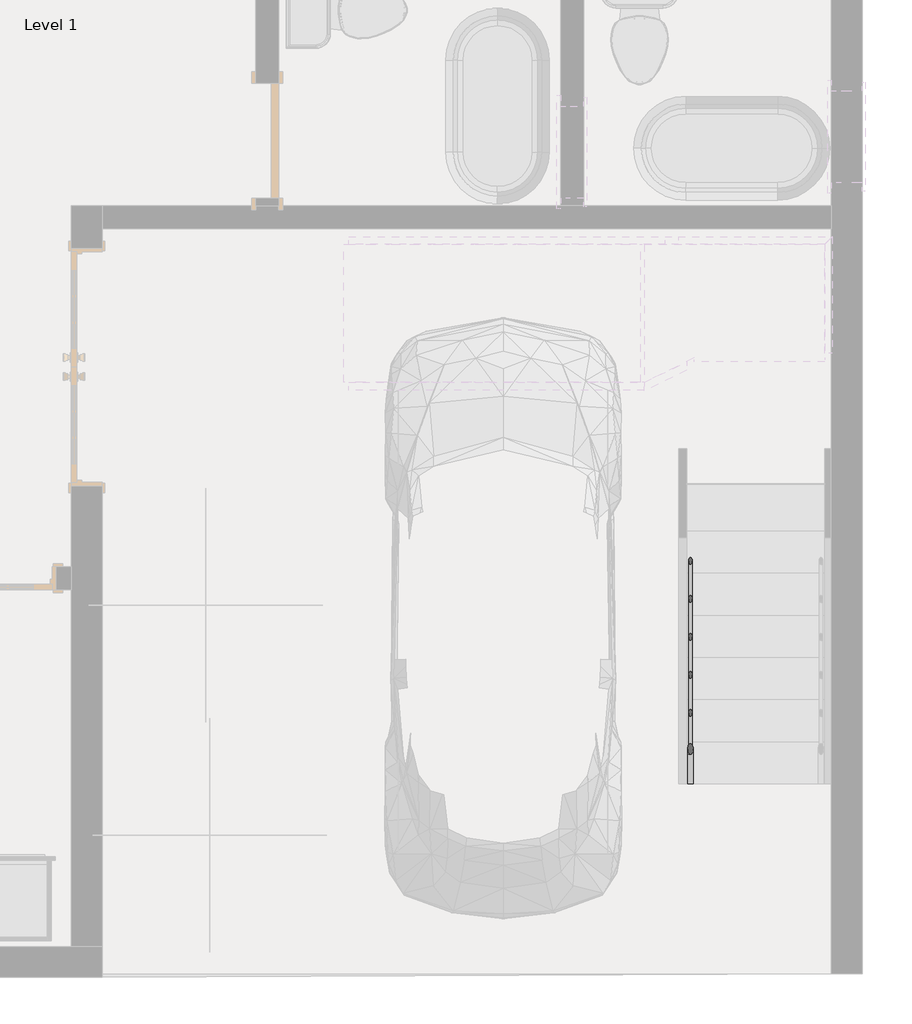
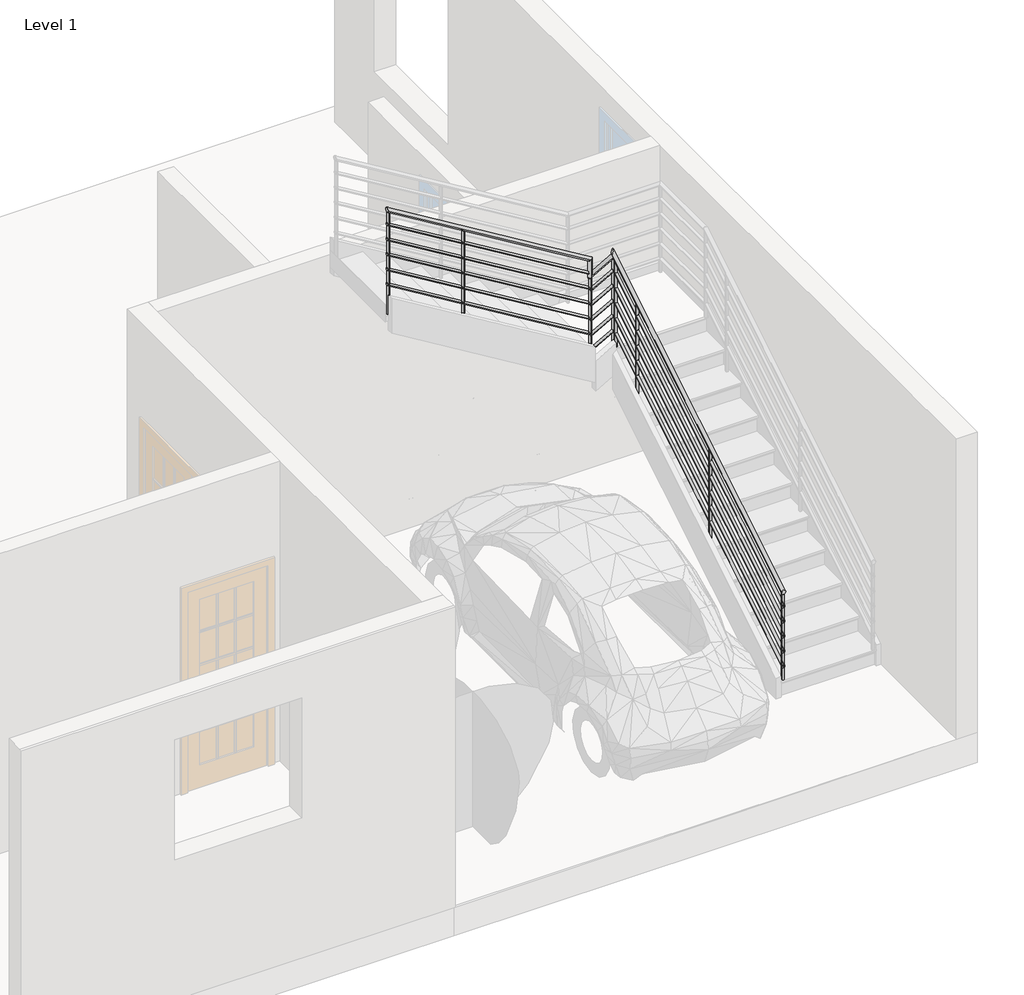
# One storey, part 3 of 5: 1 railing.
"""IFC4 building model written with IfcOpenShell, lengths in millimetres."""

from ifc_helpers import new_model, si_unit, point, frame, frame_2d, origin, place, context, project, spatial, circle_curve, ellipse_curve, trimmed, segment, composite_curve, outline, extrude, element, save
from ifc_brep_helpers import plane_surface, cylinder_surface, advanced_brep

model = new_model("IFC4")

# Units and contexts
model_context = context("Model", 3, world=origin())
ifc_project = project(units=[si_unit("LENGTHUNIT", "METRE", prefix="MILLI")], contexts=[model_context])

# Site, building, storey
site = spatial("IfcSite", under=ifc_project)
building = spatial("IfcBuilding", under=site)
storey = spatial("IfcBuildingStorey", under=building, Name="Level 1", Elevation=0.0)

# Railing
placement = place(None, origin())
element("IfcRailing", 1, ObjectType="Handrail - Pipe", at=placement, inside=storey, context=model_context, shape_type="SolidModel", body=[
    advanced_brep(
    [(-2070.9432736, 3353.09939, 1061.4577857), (-2109.0432736, 3353.09939, 1061.4577857), (-2070.9432736, 6227.2776284, 2803.3839908), (-2109.0432736, 6180.2977008, 2774.9113074)],
    [
        (0, 1, ellipse_curve(frame((-2089.9932736, 3353.09939, 1061.4577857), z_axis=(0.0, -1.0, 0.0), x_axis=(0.0, 0.0, -1.0)), 22.2755476, 19.05)),
        (1, 0, ellipse_curve(frame((-2089.9932736, 3353.09939, 1061.4577857), z_axis=(0.0, -1.0, 0.0), x_axis=(0.0, 0.0, -1.0)), 22.2755476, 19.05)),
        (2, 3, ellipse_curve(frame((-2089.9932736, 6203.7876646, 2789.1476491), z_axis=(-0.8042186020459581, 0.37062014395580417, 0.4646215115741242), x_axis=(-0.5404442051383958, -0.7813013786122838, -0.31223103130674323)), 34.1540054, 19.05)),
        (3, 2, ellipse_curve(frame((-2089.9932736, 6203.7876646, 2789.1476491), z_axis=(-0.8042186020459581, 0.37062014395580417, 0.4646215115741242), x_axis=(-0.5404442051383958, -0.7813013786122838, -0.31223103130674323)), 34.1540054, 19.05)),
        (0, 2),
        (3, 1),
    ],
    [
        plane_surface(frame((-2089.9932736, 3353.09939, 1083.7333333), z_axis=(0.0, -1.0, 0.0), x_axis=(0.0, 0.0, 1.0))),
        plane_surface(frame((-2089.9932736, 6187.918979, 2801.8058115), z_axis=(-0.8042186020459581, 0.37062014395580417, 0.4646215115741242), x_axis=(0.5943336101241835, 0.5015022017683473, 0.6286995319691712))),
        cylinder_surface(frame((-2089.9932736, 3362.9730377, 1067.4418146), z_axis=(0.0, -0.8551978315540538, -0.5183017160932851), x_axis=(-1.0, 0.0, 0.0)), 19.05),
    ],
    [
        (0, [[1, 2]]),
        (1, [[3, 4]]),
        (2, [[-1, 5, -4, 6]]),
        (2, [[-2, -6, -3, -5]]),
    ],
),
    advanced_brep(
    [(-2091.5714529, 6208.3761472, 2758.0166667), (-2116.8877776, 6153.4415743, 2758.0166667), (-2409.12329, 6052.0104202, 2758.0166667), (-2392.2923116, 6017.8296044, 2758.0166667)],
    [
        (0, 1, ellipse_curve(frame((-2104.2296153, 6180.9088608, 2758.0166667), z_axis=(0.8042186020459581, -0.37062014395580417, -0.4646215115741242), x_axis=(0.5404442051383956, 0.7813013786122838, 0.31223103130674307)), 34.1540054, 19.05)),
        (1, 0, ellipse_curve(frame((-2104.2296153, 6180.9088608, 2758.0166667), z_axis=(0.8042186020459581, -0.37062014395580417, -0.4646215115741242), x_axis=(0.5404442051383956, 0.7813013786122838, 0.31223103130674307)), 34.1540054, 19.05)),
        (2, 3, ellipse_curve(frame((-2400.7078008, 6034.9200123, 2758.0166667), z_axis=(-0.6343697273857986, -0.31237005134370305, 0.7071067811865476), x_axis=(0.6343697273857984, 0.312370051343703, 0.7071067811865476)), 26.9407684, 19.05)),
        (3, 2, ellipse_curve(frame((-2400.7078008, 6034.9200123, 2758.0166667), z_axis=(-0.6343697273857986, -0.31237005134370305, 0.7071067811865476), x_axis=(0.6343697273857984, 0.312370051343703, 0.7071067811865476)), 26.9407684, 19.05)),
        (0, 2),
        (3, 1),
    ],
    [
        plane_surface(frame((-2089.9932736, 6187.918979, 2777.0666667), z_axis=(0.8042186020459581, -0.37062014395580417, -0.4646215115741242), x_axis=(0.5943336101241835, 0.5015022017683473, 0.6286995319691712))),
        plane_surface(frame((-2383.6173929, 6043.3355015, 2777.0666667), z_axis=(-0.6343697273857987, -0.3123700513437031, 0.7071067811865477), x_axis=(0.7730297853100279, -0.2563395461339441, 0.5802714779406066))),
        cylinder_surface(frame((-2089.9932736, 6187.918979, 2758.0166667), z_axis=(0.8971342720279193, 0.44175796308944487, 0.0), x_axis=(0.44175796308944487, -0.8971342720279193, 0.0)), 19.05),
    ],
    [
        (0, [[1, 2]]),
        (1, [[3, 4]]),
        (2, [[-1, 5, -4, 6]]),
        (2, [[-2, -6, -3, -5]]),
    ],
),
    advanced_brep(
    [(-2409.12329, 6052.0104202, 2758.0166667), (-2392.2923116, 6017.8296044, 2758.0166667), (-2409.12329, 6052.0104202, 2922.9689103), (-2392.2923116, 6017.8296044, 2932.4491184)],
    [
        (0, 1, ellipse_curve(frame((-2400.7078008, 6034.9200123, 2758.0166667), z_axis=(0.6343697273857986, 0.31237005134370305, -0.7071067811865476), x_axis=(-0.6343697273857987, -0.3123700513437031, -0.7071067811865475)), 26.9407684, 19.05)),
        (1, 0, ellipse_curve(frame((-2400.7078008, 6034.9200123, 2758.0166667), z_axis=(0.6343697273857986, 0.31237005134370305, -0.7071067811865476), x_axis=(-0.6343697273857987, -0.3123700513437031, -0.7071067811865475)), 26.9407684, 19.05)),
        (2, 3, ellipse_curve(frame((-2400.7078008, 6034.9200123, 2927.7090143), z_axis=(-0.4907638352133923, 0.0, 0.8712926362862494), x_axis=(-0.8712926362862494, 0.0, -0.49076383521339195)), 21.8640663, 19.05)),
        (3, 2, ellipse_curve(frame((-2400.7078008, 6034.9200123, 2927.7090143), z_axis=(-0.4907638352133923, 0.0, 0.8712926362862494), x_axis=(-0.8712926362862494, 0.0, -0.49076383521339195)), 21.8640663, 19.05)),
        (0, 2),
        (3, 1),
    ],
    [
        plane_surface(frame((-2400.7078008, 6034.9200123, 2758.0166667), z_axis=(0.6343697273857987, 0.3123700513437031, -0.7071067811865477), x_axis=(0.7730297853100279, -0.2563395461339441, 0.5802714779406066))),
        plane_surface(frame((-2400.7078008, 6034.9200123, 2927.7090143), z_axis=(-0.4907638352133923, 0.0, 0.8712926362862494), x_axis=(0.8712926362862494, 0.0, 0.4907638352133923))),
        cylinder_surface(frame((-2400.7078008, 6034.9200123, 2758.0166667), z_axis=(0.0, 0.0, -1.0), x_axis=(0.44175796308944487, -0.8971342720279193, 0.0)), 19.05),
    ],
    [
        (0, [[1, 2]]),
        (1, [[3, 4]]),
        (2, [[-1, 5, -4, 6]]),
        (2, [[-2, -6, -3, -5]]),
    ],
),
    advanced_brep(
    [(-2400.7078008, 6053.9700123, 2927.7090143), (-2400.7078008, 6015.8700123, 2927.7090143), (-4350.5932736, 6053.9700123, 4109.4577857), (-4350.5932736, 6015.8700123, 4109.4577857)],
    [
        (0, 1, ellipse_curve(frame((-2400.7078008, 6034.9200123, 2927.7090143), z_axis=(0.4907638352133923, 0.0, -0.8712926362862494), x_axis=(0.8712926362862492, 0.0, 0.4907638352133924)), 21.8640663, 19.05)),
        (1, 0, ellipse_curve(frame((-2400.7078008, 6034.9200123, 2927.7090143), z_axis=(0.4907638352133923, 0.0, -0.8712926362862494), x_axis=(0.8712926362862492, 0.0, 0.4907638352133924)), 21.8640663, 19.05)),
        (2, 3, ellipse_curve(frame((-4350.5932736, 6034.9200123, 4109.4577857), z_axis=(-1.0, 0.0, 0.0), x_axis=(0.0, 0.0, -1.0)), 22.2755476, 19.05)),
        (3, 2, ellipse_curve(frame((-4350.5932736, 6034.9200123, 4109.4577857), z_axis=(-1.0, 0.0, 0.0), x_axis=(0.0, 0.0, -1.0)), 22.2755476, 19.05)),
        (0, 2),
        (3, 1),
    ],
    [
        plane_surface(frame((-2381.6578008, 6034.9200123, 2938.4391074), z_axis=(0.4907638352133923, 0.0, -0.8712926362862494), x_axis=(0.8712926362862494, 0.0, 0.4907638352133923))),
        plane_surface(frame((-4350.5932736, 6034.9200123, 4131.7333333), z_axis=(-1.0, 0.0, 0.0), x_axis=(0.0, -1.0, 0.0))),
        cylinder_surface(frame((-2391.5314485, 6034.9200123, 2922.1475887), z_axis=(0.855197831554054, 0.0, -0.5183017160932848), x_axis=(0.0, -1.0, 0.0)), 19.05),
    ],
    [
        (0, [[1, 2]]),
        (1, [[3, 4]]),
        (2, [[-1, 5, -4, 6]]),
        (2, [[-2, -6, -3, -5]]),
    ],
),
    advanced_brep(
    [(-2077.2932736, 3353.09939, 916.4829683), (-2102.6932736, 3353.09939, 916.4829683), (-2077.2932736, 6150.6474924, 2611.9666667), (-2102.6932736, 6150.6474924, 2611.9666667), (-2077.2932736, 6208.3287735, 2611.9666667), (-2102.6932736, 6167.5091845, 2611.9666667), (-2400.7078008, 6049.0761987, 2611.9666667), (-2400.7078008, 6020.7638259, 2611.9666667)],
    [
        (0, 1, ellipse_curve(frame((-2089.9932736, 3353.09939, 916.4829683), z_axis=(0.0, -1.0, 0.0), x_axis=(0.0, 0.0, -1.0)), 14.8503651, 12.7)),
        (1, 0, ellipse_curve(frame((-2089.9932736, 3353.09939, 916.4829683), z_axis=(0.0, -1.0, 0.0), x_axis=(0.0, 0.0, -1.0)), 14.8503651, 12.7)),
        (0, 2),
        (2, 3, ellipse_curve(frame((-2089.9932736, 6150.6474924, 2611.9666667), z_axis=(0.0, -0.9631193673564181, -0.26907449567540415), x_axis=(0.0, 0.26907449567540453, -0.9631193673564179)), 13.1863198, 12.7)),
        (3, 1),
        (3, 2, ellipse_curve(frame((-2089.9932736, 6150.6474924, 2611.9666667), z_axis=(0.0, -0.9631193673564181, -0.26907449567540415), x_axis=(0.0, 0.26907449567540453, -0.9631193673564179)), 13.1863198, 12.7)),
        (2, 4),
        (4, 5, ellipse_curve(frame((-2089.9932736, 6187.918979, 2611.9666667), z_axis=(0.849045924284854, -0.5283190498697528, 0.0), x_axis=(-0.5283190498697528, -0.8490459242848537, 0.0)), 24.0385048, 12.7)),
        (5, 3),
        (5, 4, ellipse_curve(frame((-2089.9932736, 6187.918979, 2611.9666667), z_axis=(0.849045924284854, -0.5283190498697528, 0.0), x_axis=(-0.5283190498697528, -0.8490459242848537, 0.0)), 24.0385048, 12.7)),
        (6, 7, ellipse_curve(frame((-2400.7078008, 6034.9200123, 2611.9666667), z_axis=(-1.0, 0.0, 0.0), x_axis=(0.0, 1.0, 0.0)), 14.1561864, 12.7)),
        (7, 6, ellipse_curve(frame((-2400.7078008, 6034.9200123, 2611.9666667), z_axis=(-1.0, 0.0, 0.0), x_axis=(0.0, 1.0, 0.0)), 14.1561864, 12.7)),
        (4, 6),
        (7, 5),
    ],
    [
        plane_surface(frame((-2089.9932736, 3353.09939, 931.3333333), z_axis=(0.0, -1.0, 0.0), x_axis=(0.0, 0.0, 1.0))),
        cylinder_surface(frame((-2089.9932736, 3359.6818218, 920.4723209), z_axis=(0.0, -0.8551978315540539, -0.518301716093285), x_axis=(-1.0, 0.0, 0.0)), 12.7),
        cylinder_surface(frame((-2089.9932736, 6147.09939, 2611.9666667), z_axis=(0.0, -1.0, 0.0), x_axis=(-1.0, 0.0, 0.0)), 12.7),
        plane_surface(frame((-2400.7078008, 6034.9200123, 2624.6666667), z_axis=(-1.0, 0.0, 0.0), x_axis=(0.0, -1.0, 0.0))),
        cylinder_surface(frame((-2089.9932736, 6187.918979, 2611.9666667), z_axis=(0.8971342720279194, 0.4417579630894449, 0.0), x_axis=(0.4417579630894449, -0.8971342720279194, 0.0)), 12.7),
    ],
    [
        (0, [[1, 2]]),
        (1, [[-1, 3, 4, 5]]),
        (1, [[-2, -5, 6, -3]]),
        (2, [[-4, 7, 8, 9]]),
        (2, [[-6, -9, 10, -7]]),
        (3, [[11, 12]]),
        (4, [[-8, 13, -12, 14]]),
        (4, [[-10, -14, -11, -13]]),
    ],
),
    advanced_brep(
    [(-2400.7078008, 6047.6200123, 2782.7341969), (-2400.7078008, 6022.2200123, 2782.7341969), (-4350.5932736, 6047.6200123, 3964.4829683), (-4350.5932736, 6022.2200123, 3964.4829683)],
    [
        (0, 1, ellipse_curve(frame((-2400.7078008, 6034.9200123, 2782.7341969), z_axis=(1.0, 0.0, 0.0), x_axis=(0.0, 0.0, -1.0)), 14.8503651, 12.7)),
        (1, 0, ellipse_curve(frame((-2400.7078008, 6034.9200123, 2782.7341969), z_axis=(1.0, 0.0, 0.0), x_axis=(0.0, 0.0, -1.0)), 14.8503651, 12.7)),
        (2, 3, ellipse_curve(frame((-4350.5932736, 6034.9200123, 3964.4829683), z_axis=(-1.0, 0.0, 0.0), x_axis=(0.0, 0.0, -1.0)), 14.8503651, 12.7)),
        (3, 2, ellipse_curve(frame((-4350.5932736, 6034.9200123, 3964.4829683), z_axis=(-1.0, 0.0, 0.0), x_axis=(0.0, 0.0, -1.0)), 14.8503651, 12.7)),
        (0, 2),
        (3, 1),
    ],
    [
        plane_surface(frame((-2400.7078008, 6034.9200123, 2797.5845619), z_axis=(1.0, 0.0, 0.0), x_axis=(0.0, -1.0, 0.0))),
        plane_surface(frame((-4350.5932736, 6034.9200123, 3979.3333333), z_axis=(-1.0, 0.0, 0.0), x_axis=(0.0, -1.0, 0.0))),
        cylinder_surface(frame((-2407.2902326, 6034.9200123, 2786.7235495), z_axis=(0.855197831554054, 0.0, -0.5183017160932848), x_axis=(0.0, -1.0, 0.0)), 12.7),
    ],
    [
        (0, [[1, 2]]),
        (1, [[3, 4]]),
        (2, [[-1, 5, -4, 6]]),
        (2, [[-2, -6, -3, -5]]),
    ],
),
    advanced_brep(
    [(-2077.2932736, 3353.09939, 764.0829683), (-2102.6932736, 3353.09939, 764.0829683), (-2077.2932736, 6150.6474924, 2459.5666667), (-2102.6932736, 6150.6474924, 2459.5666667), (-2077.2932736, 6208.3287735, 2459.5666667), (-2102.6932736, 6167.5091845, 2459.5666667), (-2400.7078008, 6049.0761987, 2459.5666667), (-2400.7078008, 6020.7638259, 2459.5666667)],
    [
        (0, 1, ellipse_curve(frame((-2089.9932736, 3353.09939, 764.0829683), z_axis=(0.0, -1.0, 0.0), x_axis=(0.0, 0.0, -1.0)), 14.8503651, 12.7)),
        (1, 0, ellipse_curve(frame((-2089.9932736, 3353.09939, 764.0829683), z_axis=(0.0, -1.0, 0.0), x_axis=(0.0, 0.0, -1.0)), 14.8503651, 12.7)),
        (0, 2),
        (2, 3, ellipse_curve(frame((-2089.9932736, 6150.6474924, 2459.5666667), z_axis=(0.0, -0.9631193673564181, -0.26907449567540415), x_axis=(0.0, 0.26907449567540453, -0.9631193673564179)), 13.1863198, 12.7)),
        (3, 1),
        (3, 2, ellipse_curve(frame((-2089.9932736, 6150.6474924, 2459.5666667), z_axis=(0.0, -0.9631193673564181, -0.26907449567540415), x_axis=(0.0, 0.26907449567540453, -0.9631193673564179)), 13.1863198, 12.7)),
        (2, 4),
        (4, 5, ellipse_curve(frame((-2089.9932736, 6187.918979, 2459.5666667), z_axis=(0.849045924284854, -0.5283190498697528, 0.0), x_axis=(-0.5283190498697528, -0.8490459242848537, 0.0)), 24.0385048, 12.7)),
        (5, 3),
        (5, 4, ellipse_curve(frame((-2089.9932736, 6187.918979, 2459.5666667), z_axis=(0.849045924284854, -0.5283190498697528, 0.0), x_axis=(-0.5283190498697528, -0.8490459242848537, 0.0)), 24.0385048, 12.7)),
        (6, 7, ellipse_curve(frame((-2400.7078008, 6034.9200123, 2459.5666667), z_axis=(-1.0, 0.0, 0.0), x_axis=(0.0, 1.0, 0.0)), 14.1561864, 12.7)),
        (7, 6, ellipse_curve(frame((-2400.7078008, 6034.9200123, 2459.5666667), z_axis=(-1.0, 0.0, 0.0), x_axis=(0.0, 1.0, 0.0)), 14.1561864, 12.7)),
        (4, 6),
        (7, 5),
    ],
    [
        plane_surface(frame((-2089.9932736, 3353.09939, 778.9333333), z_axis=(0.0, -1.0, 0.0), x_axis=(0.0, 0.0, 1.0))),
        cylinder_surface(frame((-2089.9932736, 3359.6818218, 768.0723209), z_axis=(0.0, -0.8551978315540539, -0.518301716093285), x_axis=(-1.0, 0.0, 0.0)), 12.7),
        cylinder_surface(frame((-2089.9932736, 6147.09939, 2459.5666667), z_axis=(0.0, -1.0, 0.0), x_axis=(-1.0, 0.0, 0.0)), 12.7),
        plane_surface(frame((-2400.7078008, 6034.9200123, 2472.2666667), z_axis=(-1.0, 0.0, 0.0), x_axis=(0.0, -1.0, 0.0))),
        cylinder_surface(frame((-2089.9932736, 6187.918979, 2459.5666667), z_axis=(0.8971342720279194, 0.4417579630894449, 0.0), x_axis=(0.4417579630894449, -0.8971342720279194, 0.0)), 12.7),
    ],
    [
        (0, [[1, 2]]),
        (1, [[-1, 3, 4, 5]]),
        (1, [[-2, -5, 6, -3]]),
        (2, [[-4, 7, 8, 9]]),
        (2, [[-6, -9, 10, -7]]),
        (3, [[11, 12]]),
        (4, [[-8, 13, -12, 14]]),
        (4, [[-10, -14, -11, -13]]),
    ],
),
    advanced_brep(
    [(-2400.7078008, 6047.6200123, 2630.3341969), (-2400.7078008, 6022.2200123, 2630.3341969), (-4350.5932736, 6047.6200123, 3812.0829683), (-4350.5932736, 6022.2200123, 3812.0829683)],
    [
        (0, 1, ellipse_curve(frame((-2400.7078008, 6034.9200123, 2630.3341969), z_axis=(1.0, 0.0, 0.0), x_axis=(0.0, 0.0, -1.0)), 14.8503651, 12.7)),
        (1, 0, ellipse_curve(frame((-2400.7078008, 6034.9200123, 2630.3341969), z_axis=(1.0, 0.0, 0.0), x_axis=(0.0, 0.0, -1.0)), 14.8503651, 12.7)),
        (2, 3, ellipse_curve(frame((-4350.5932736, 6034.9200123, 3812.0829683), z_axis=(-1.0, 0.0, 0.0), x_axis=(0.0, 0.0, -1.0)), 14.8503651, 12.7)),
        (3, 2, ellipse_curve(frame((-4350.5932736, 6034.9200123, 3812.0829683), z_axis=(-1.0, 0.0, 0.0), x_axis=(0.0, 0.0, -1.0)), 14.8503651, 12.7)),
        (0, 2),
        (3, 1),
    ],
    [
        plane_surface(frame((-2400.7078008, 6034.9200123, 2645.1845619), z_axis=(1.0, 0.0, 0.0), x_axis=(0.0, -1.0, 0.0))),
        plane_surface(frame((-4350.5932736, 6034.9200123, 3826.9333333), z_axis=(-1.0, 0.0, 0.0), x_axis=(0.0, -1.0, 0.0))),
        cylinder_surface(frame((-2407.2902326, 6034.9200123, 2634.3235495), z_axis=(0.855197831554054, 0.0, -0.5183017160932848), x_axis=(0.0, -1.0, 0.0)), 12.7),
    ],
    [
        (0, [[1, 2]]),
        (1, [[3, 4]]),
        (2, [[-1, 5, -4, 6]]),
        (2, [[-2, -6, -3, -5]]),
    ],
),
    advanced_brep(
    [(-2077.2932736, 3353.09939, 611.6829683), (-2102.6932736, 3353.09939, 611.6829683), (-2077.2932736, 6150.6474924, 2307.1666667), (-2102.6932736, 6150.6474924, 2307.1666667), (-2077.2932736, 6208.3287735, 2307.1666667), (-2102.6932736, 6167.5091845, 2307.1666667), (-2400.7078008, 6049.0761987, 2307.1666667), (-2400.7078008, 6020.7638259, 2307.1666667)],
    [
        (0, 1, ellipse_curve(frame((-2089.9932736, 3353.09939, 611.6829683), z_axis=(0.0, -1.0, 0.0), x_axis=(0.0, 0.0, -1.0)), 14.8503651, 12.7)),
        (1, 0, ellipse_curve(frame((-2089.9932736, 3353.09939, 611.6829683), z_axis=(0.0, -1.0, 0.0), x_axis=(0.0, 0.0, -1.0)), 14.8503651, 12.7)),
        (0, 2),
        (2, 3, ellipse_curve(frame((-2089.9932736, 6150.6474924, 2307.1666667), z_axis=(0.0, -0.9631193673564181, -0.26907449567540415), x_axis=(0.0, 0.26907449567540453, -0.9631193673564179)), 13.1863198, 12.7)),
        (3, 1),
        (3, 2, ellipse_curve(frame((-2089.9932736, 6150.6474924, 2307.1666667), z_axis=(0.0, -0.9631193673564181, -0.26907449567540415), x_axis=(0.0, 0.26907449567540453, -0.9631193673564179)), 13.1863198, 12.7)),
        (2, 4),
        (4, 5, ellipse_curve(frame((-2089.9932736, 6187.918979, 2307.1666667), z_axis=(0.849045924284854, -0.5283190498697528, 0.0), x_axis=(-0.5283190498697528, -0.8490459242848537, 0.0)), 24.0385048, 12.7)),
        (5, 3),
        (5, 4, ellipse_curve(frame((-2089.9932736, 6187.918979, 2307.1666667), z_axis=(0.849045924284854, -0.5283190498697528, 0.0), x_axis=(-0.5283190498697528, -0.8490459242848537, 0.0)), 24.0385048, 12.7)),
        (6, 7, ellipse_curve(frame((-2400.7078008, 6034.9200123, 2307.1666667), z_axis=(-1.0, 0.0, 0.0), x_axis=(0.0, 1.0, 0.0)), 14.1561864, 12.7)),
        (7, 6, ellipse_curve(frame((-2400.7078008, 6034.9200123, 2307.1666667), z_axis=(-1.0, 0.0, 0.0), x_axis=(0.0, 1.0, 0.0)), 14.1561864, 12.7)),
        (4, 6),
        (7, 5),
    ],
    [
        plane_surface(frame((-2089.9932736, 3353.09939, 626.5333333), z_axis=(0.0, -1.0, 0.0), x_axis=(0.0, 0.0, 1.0))),
        cylinder_surface(frame((-2089.9932736, 3359.6818218, 615.6723209), z_axis=(0.0, -0.8551978315540539, -0.518301716093285), x_axis=(-1.0, 0.0, 0.0)), 12.7),
        cylinder_surface(frame((-2089.9932736, 6147.09939, 2307.1666667), z_axis=(0.0, -1.0, 0.0), x_axis=(-1.0, 0.0, 0.0)), 12.7),
        plane_surface(frame((-2400.7078008, 6034.9200123, 2319.8666667), z_axis=(-1.0, 0.0, 0.0), x_axis=(0.0, -1.0, 0.0))),
        cylinder_surface(frame((-2089.9932736, 6187.918979, 2307.1666667), z_axis=(0.8971342720279194, 0.4417579630894449, 0.0), x_axis=(0.4417579630894449, -0.8971342720279194, 0.0)), 12.7),
    ],
    [
        (0, [[1, 2]]),
        (1, [[-1, 3, 4, 5]]),
        (1, [[-2, -5, 6, -3]]),
        (2, [[-4, 7, 8, 9]]),
        (2, [[-6, -9, 10, -7]]),
        (3, [[11, 12]]),
        (4, [[-8, 13, -12, 14]]),
        (4, [[-10, -14, -11, -13]]),
    ],
),
    advanced_brep(
    [(-2400.7078008, 6047.6200123, 2477.9341969), (-2400.7078008, 6022.2200123, 2477.9341969), (-4350.5932736, 6047.6200123, 3659.6829683), (-4350.5932736, 6022.2200123, 3659.6829683)],
    [
        (0, 1, ellipse_curve(frame((-2400.7078008, 6034.9200123, 2477.9341969), z_axis=(1.0, 0.0, 0.0), x_axis=(0.0, 0.0, -1.0)), 14.8503651, 12.7)),
        (1, 0, ellipse_curve(frame((-2400.7078008, 6034.9200123, 2477.9341969), z_axis=(1.0, 0.0, 0.0), x_axis=(0.0, 0.0, -1.0)), 14.8503651, 12.7)),
        (2, 3, ellipse_curve(frame((-4350.5932736, 6034.9200123, 3659.6829683), z_axis=(-1.0, 0.0, 0.0), x_axis=(0.0, 0.0, -1.0)), 14.8503651, 12.7)),
        (3, 2, ellipse_curve(frame((-4350.5932736, 6034.9200123, 3659.6829683), z_axis=(-1.0, 0.0, 0.0), x_axis=(0.0, 0.0, -1.0)), 14.8503651, 12.7)),
        (0, 2),
        (3, 1),
    ],
    [
        plane_surface(frame((-2400.7078008, 6034.9200123, 2492.7845619), z_axis=(1.0, 0.0, 0.0), x_axis=(0.0, -1.0, 0.0))),
        plane_surface(frame((-4350.5932736, 6034.9200123, 3674.5333333), z_axis=(-1.0, 0.0, 0.0), x_axis=(0.0, -1.0, 0.0))),
        cylinder_surface(frame((-2407.2902326, 6034.9200123, 2481.9235495), z_axis=(0.855197831554054, 0.0, -0.5183017160932848), x_axis=(0.0, -1.0, 0.0)), 12.7),
    ],
    [
        (0, [[1, 2]]),
        (1, [[3, 4]]),
        (2, [[-1, 5, -4, 6]]),
        (2, [[-2, -6, -3, -5]]),
    ],
),
    advanced_brep(
    [(-2077.2932736, 3353.09939, 459.2829683), (-2102.6932736, 3353.09939, 459.2829683), (-2077.2932736, 6150.6474924, 2154.7666667), (-2102.6932736, 6150.6474924, 2154.7666667), (-2077.2932736, 6208.3287735, 2154.7666667), (-2102.6932736, 6167.5091845, 2154.7666667), (-2400.7078008, 6049.0761987, 2154.7666667), (-2400.7078008, 6020.7638259, 2154.7666667)],
    [
        (0, 1, ellipse_curve(frame((-2089.9932736, 3353.09939, 459.2829683), z_axis=(0.0, -1.0, 0.0), x_axis=(0.0, 0.0, -1.0)), 14.8503651, 12.7)),
        (1, 0, ellipse_curve(frame((-2089.9932736, 3353.09939, 459.2829683), z_axis=(0.0, -1.0, 0.0), x_axis=(0.0, 0.0, -1.0)), 14.8503651, 12.7)),
        (0, 2),
        (2, 3, ellipse_curve(frame((-2089.9932736, 6150.6474924, 2154.7666667), z_axis=(0.0, -0.9631193673564181, -0.26907449567540415), x_axis=(0.0, 0.26907449567540453, -0.9631193673564179)), 13.1863198, 12.7)),
        (3, 1),
        (3, 2, ellipse_curve(frame((-2089.9932736, 6150.6474924, 2154.7666667), z_axis=(0.0, -0.9631193673564181, -0.26907449567540415), x_axis=(0.0, 0.26907449567540453, -0.9631193673564179)), 13.1863198, 12.7)),
        (2, 4),
        (4, 5, ellipse_curve(frame((-2089.9932736, 6187.918979, 2154.7666667), z_axis=(0.849045924284854, -0.5283190498697528, 0.0), x_axis=(-0.5283190498697528, -0.8490459242848537, 0.0)), 24.0385048, 12.7)),
        (5, 3),
        (5, 4, ellipse_curve(frame((-2089.9932736, 6187.918979, 2154.7666667), z_axis=(0.849045924284854, -0.5283190498697528, 0.0), x_axis=(-0.5283190498697528, -0.8490459242848537, 0.0)), 24.0385048, 12.7)),
        (6, 7, ellipse_curve(frame((-2400.7078008, 6034.9200123, 2154.7666667), z_axis=(-1.0, 0.0, 0.0), x_axis=(0.0, 1.0, 0.0)), 14.1561864, 12.7)),
        (7, 6, ellipse_curve(frame((-2400.7078008, 6034.9200123, 2154.7666667), z_axis=(-1.0, 0.0, 0.0), x_axis=(0.0, 1.0, 0.0)), 14.1561864, 12.7)),
        (4, 6),
        (7, 5),
    ],
    [
        plane_surface(frame((-2089.9932736, 3353.09939, 474.1333333), z_axis=(0.0, -1.0, 0.0), x_axis=(0.0, 0.0, 1.0))),
        cylinder_surface(frame((-2089.9932736, 3359.6818218, 463.2723209), z_axis=(0.0, -0.8551978315540539, -0.518301716093285), x_axis=(-1.0, 0.0, 0.0)), 12.7),
        cylinder_surface(frame((-2089.9932736, 6147.09939, 2154.7666667), z_axis=(0.0, -1.0, 0.0), x_axis=(-1.0, 0.0, 0.0)), 12.7),
        plane_surface(frame((-2400.7078008, 6034.9200123, 2167.4666667), z_axis=(-1.0, 0.0, 0.0), x_axis=(0.0, -1.0, 0.0))),
        cylinder_surface(frame((-2089.9932736, 6187.918979, 2154.7666667), z_axis=(0.8971342720279194, 0.4417579630894449, 0.0), x_axis=(0.4417579630894449, -0.8971342720279194, 0.0)), 12.7),
    ],
    [
        (0, [[1, 2]]),
        (1, [[-1, 3, 4, 5]]),
        (1, [[-2, -5, 6, -3]]),
        (2, [[-4, 7, 8, 9]]),
        (2, [[-6, -9, 10, -7]]),
        (3, [[11, 12]]),
        (4, [[-8, 13, -12, 14]]),
        (4, [[-10, -14, -11, -13]]),
    ],
),
    advanced_brep(
    [(-2400.7078008, 6047.6200123, 2325.5341969), (-2400.7078008, 6022.2200123, 2325.5341969), (-4350.5932736, 6047.6200123, 3507.2829683), (-4350.5932736, 6022.2200123, 3507.2829683)],
    [
        (0, 1, ellipse_curve(frame((-2400.7078008, 6034.9200123, 2325.5341969), z_axis=(1.0, 0.0, 0.0), x_axis=(0.0, 0.0, -1.0)), 14.8503651, 12.7)),
        (1, 0, ellipse_curve(frame((-2400.7078008, 6034.9200123, 2325.5341969), z_axis=(1.0, 0.0, 0.0), x_axis=(0.0, 0.0, -1.0)), 14.8503651, 12.7)),
        (2, 3, ellipse_curve(frame((-4350.5932736, 6034.9200123, 3507.2829683), z_axis=(-1.0, 0.0, 0.0), x_axis=(0.0, 0.0, -1.0)), 14.8503651, 12.7)),
        (3, 2, ellipse_curve(frame((-4350.5932736, 6034.9200123, 3507.2829683), z_axis=(-1.0, 0.0, 0.0), x_axis=(0.0, 0.0, -1.0)), 14.8503651, 12.7)),
        (0, 2),
        (3, 1),
    ],
    [
        plane_surface(frame((-2400.7078008, 6034.9200123, 2340.3845619), z_axis=(1.0, 0.0, 0.0), x_axis=(0.0, -1.0, 0.0))),
        plane_surface(frame((-4350.5932736, 6034.9200123, 3522.1333333), z_axis=(-1.0, 0.0, 0.0), x_axis=(0.0, -1.0, 0.0))),
        cylinder_surface(frame((-2407.2902326, 6034.9200123, 2329.5235495), z_axis=(0.855197831554054, 0.0, -0.5183017160932847), x_axis=(0.0, -1.0, 0.0)), 12.7),
    ],
    [
        (0, [[1, 2]]),
        (1, [[3, 4]]),
        (2, [[-1, 5, -4, 6]]),
        (2, [[-2, -6, -3, -5]]),
    ],
),
    advanced_brep(
    [(-2077.2932736, 3353.09939, 306.8829683), (-2102.6932736, 3353.09939, 306.8829683), (-2077.2932736, 6150.6474924, 2002.3666667), (-2102.6932736, 6150.6474924, 2002.3666667), (-2077.2932736, 6208.3287735, 2002.3666667), (-2102.6932736, 6167.5091845, 2002.3666667), (-2400.7078008, 6049.0761987, 2002.3666667), (-2400.7078008, 6020.7638259, 2002.3666667)],
    [
        (0, 1, ellipse_curve(frame((-2089.9932736, 3353.09939, 306.8829683), z_axis=(0.0, -1.0, 0.0), x_axis=(0.0, 0.0, -1.0)), 14.8503651, 12.7)),
        (1, 0, ellipse_curve(frame((-2089.9932736, 3353.09939, 306.8829683), z_axis=(0.0, -1.0, 0.0), x_axis=(0.0, 0.0, -1.0)), 14.8503651, 12.7)),
        (0, 2),
        (2, 3, ellipse_curve(frame((-2089.9932736, 6150.6474924, 2002.3666667), z_axis=(0.0, -0.9631193673564181, -0.26907449567540415), x_axis=(0.0, 0.26907449567540453, -0.9631193673564179)), 13.1863198, 12.7)),
        (3, 1),
        (3, 2, ellipse_curve(frame((-2089.9932736, 6150.6474924, 2002.3666667), z_axis=(0.0, -0.9631193673564181, -0.26907449567540415), x_axis=(0.0, 0.26907449567540453, -0.9631193673564179)), 13.1863198, 12.7)),
        (2, 4),
        (4, 5, ellipse_curve(frame((-2089.9932736, 6187.918979, 2002.3666667), z_axis=(0.849045924284854, -0.5283190498697528, 0.0), x_axis=(-0.5283190498697528, -0.8490459242848537, 0.0)), 24.0385048, 12.7)),
        (5, 3),
        (5, 4, ellipse_curve(frame((-2089.9932736, 6187.918979, 2002.3666667), z_axis=(0.849045924284854, -0.5283190498697528, 0.0), x_axis=(-0.5283190498697528, -0.8490459242848537, 0.0)), 24.0385048, 12.7)),
        (6, 7, ellipse_curve(frame((-2400.7078008, 6034.9200123, 2002.3666667), z_axis=(-1.0, 0.0, 0.0), x_axis=(0.0, 1.0, 0.0)), 14.1561864, 12.7)),
        (7, 6, ellipse_curve(frame((-2400.7078008, 6034.9200123, 2002.3666667), z_axis=(-1.0, 0.0, 0.0), x_axis=(0.0, 1.0, 0.0)), 14.1561864, 12.7)),
        (4, 6),
        (7, 5),
    ],
    [
        plane_surface(frame((-2089.9932736, 3353.09939, 321.7333333), z_axis=(0.0, -1.0, 0.0), x_axis=(0.0, 0.0, 1.0))),
        cylinder_surface(frame((-2089.9932736, 3359.6818218, 310.8723209), z_axis=(0.0, -0.8551978315540539, -0.518301716093285), x_axis=(-1.0, 0.0, 0.0)), 12.7),
        cylinder_surface(frame((-2089.9932736, 6147.09939, 2002.3666667), z_axis=(0.0, -1.0, 0.0), x_axis=(-1.0, 0.0, 0.0)), 12.7),
        plane_surface(frame((-2400.7078008, 6034.9200123, 2015.0666667), z_axis=(-1.0, 0.0, 0.0), x_axis=(0.0, -1.0, 0.0))),
        cylinder_surface(frame((-2089.9932736, 6187.918979, 2002.3666667), z_axis=(0.8971342720279194, 0.4417579630894449, 0.0), x_axis=(0.4417579630894449, -0.8971342720279194, 0.0)), 12.7),
    ],
    [
        (0, [[1, 2]]),
        (1, [[-1, 3, 4, 5]]),
        (1, [[-2, -5, 6, -3]]),
        (2, [[-4, 7, 8, 9]]),
        (2, [[-6, -9, 10, -7]]),
        (3, [[11, 12]]),
        (4, [[-8, 13, -12, 14]]),
        (4, [[-10, -14, -11, -13]]),
    ],
),
    advanced_brep(
    [(-2400.7078008, 6047.6200123, 2173.1341969), (-2400.7078008, 6022.2200123, 2173.1341969), (-4350.5932736, 6047.6200123, 3354.8829683), (-4350.5932736, 6022.2200123, 3354.8829683)],
    [
        (0, 1, ellipse_curve(frame((-2400.7078008, 6034.9200123, 2173.1341969), z_axis=(1.0, 0.0, 0.0), x_axis=(0.0, 0.0, -1.0)), 14.8503651, 12.7)),
        (1, 0, ellipse_curve(frame((-2400.7078008, 6034.9200123, 2173.1341969), z_axis=(1.0, 0.0, 0.0), x_axis=(0.0, 0.0, -1.0)), 14.8503651, 12.7)),
        (2, 3, ellipse_curve(frame((-4350.5932736, 6034.9200123, 3354.8829683), z_axis=(-1.0, 0.0, 0.0), x_axis=(0.0, 0.0, -1.0)), 14.8503651, 12.7)),
        (3, 2, ellipse_curve(frame((-4350.5932736, 6034.9200123, 3354.8829683), z_axis=(-1.0, 0.0, 0.0), x_axis=(0.0, 0.0, -1.0)), 14.8503651, 12.7)),
        (0, 2),
        (3, 1),
    ],
    [
        plane_surface(frame((-2400.7078008, 6034.9200123, 2187.9845619), z_axis=(1.0, 0.0, 0.0), x_axis=(0.0, -1.0, 0.0))),
        plane_surface(frame((-4350.5932736, 6034.9200123, 3369.7333333), z_axis=(-1.0, 0.0, 0.0), x_axis=(0.0, -1.0, 0.0))),
        cylinder_surface(frame((-2407.2902326, 6034.9200123, 2177.1235495), z_axis=(0.855197831554054, 0.0, -0.5183017160932847), x_axis=(0.0, -1.0, 0.0)), 12.7),
    ],
    [
        (0, [[1, 2]]),
        (1, [[3, 4]]),
        (2, [[-1, 5, -4, 6]]),
        (2, [[-2, -6, -3, -5]]),
    ],
),
    advanced_brep(
    [(-3619.9078008, 6022.2200123, 3644.3425577), (-3619.9078008, 6047.6200123, 3644.3425577), (-3619.9078008, 6047.6200123, 2709.3333333), (-3619.9078008, 6022.2200123, 2709.3333333)],
    [
        (0, 1, ellipse_curve(frame((-3619.9078008, 6034.9200123, 3644.3425577), z_axis=(-0.5183017160932833, 0.0, -0.8551978315540549), x_axis=(-0.855197831554055, 0.0, 0.518301716093283)), 14.8503651, 12.7)),
        (1, 2),
        (2, 3, circle_curve(frame((-3619.9078008, 6034.9200123, 2709.3333333), z_axis=(0.0, 0.0, 1.0), x_axis=(0.0, 1.0, 0.0)), 12.7)),
        (3, 0),
        (3, 2, circle_curve(frame((-3619.9078008, 6034.9200123, 2709.3333333), z_axis=(0.0, 0.0, 1.0), x_axis=(0.0, 1.0, 0.0)), 12.7)),
        (1, 0, ellipse_curve(frame((-3619.9078008, 6034.9200123, 3644.3425577), z_axis=(-0.5183017160932833, 0.0, -0.8551978315540549), x_axis=(-0.855197831554055, 0.0, 0.518301716093283)), 14.8503651, 12.7)),
    ],
    [
        cylinder_surface(frame((-3619.9078008, 6034.9200123, 2480.7333333), z_axis=(0.0, 0.0, 1.0), x_axis=(0.0, 1.0, 0.0)), 12.7),
        plane_surface(frame((-3645.3078008, 6060.3200123, 3659.7364971), z_axis=(0.5183017160932833, 0.0, 0.8551978315540549), x_axis=(0.0, -1.0, 0.0))),
        plane_surface(frame((-3594.5078008, 6060.3200123, 2709.3333333), z_axis=(0.0, 0.0, -1.0), x_axis=(0.0, -1.0, 0.0))),
    ],
    [
        (0, [[1, 2, 3, 4]]),
        (0, [[5, -2, 6, -4]]),
        (1, [[-6, -1]]),
        (2, [[-5, -3]]),
    ],
),
    advanced_brep(
    [(-2102.6932736, 5791.49939, 2517.00042), (-2077.2932736, 5791.49939, 2517.00042), (-2077.2932736, 5791.49939, 1524.0), (-2102.6932736, 5791.49939, 1524.0)],
    [
        (0, 1, ellipse_curve(frame((-2089.9932736, 5791.49939, 2517.00042), z_axis=(0.0, 0.5183017160932833, -0.8551978315540549), x_axis=(0.0, 0.855197831554055, 0.518301716093283)), 14.8503651, 12.7)),
        (1, 2),
        (2, 3, circle_curve(frame((-2089.9932736, 5791.49939, 1524.0), z_axis=(0.0, 0.0, 1.0), x_axis=(1.0, 0.0, 0.0)), 12.7)),
        (3, 0),
        (3, 2, circle_curve(frame((-2089.9932736, 5791.49939, 1524.0), z_axis=(0.0, 0.0, 1.0), x_axis=(1.0, 0.0, 0.0)), 12.7)),
        (1, 0, ellipse_curve(frame((-2089.9932736, 5791.49939, 2517.00042), z_axis=(0.0, 0.5183017160932833, -0.8551978315540549), x_axis=(0.0, 0.855197831554055, 0.518301716093283)), 14.8503651, 12.7)),
    ],
    [
        cylinder_surface(frame((-2089.9932736, 5791.49939, 1295.4), z_axis=(0.0, 0.0, 1.0), x_axis=(1.0, 0.0, 0.0)), 12.7),
        plane_surface(frame((-2064.5932736, 5816.89939, 2532.3943594), z_axis=(0.0, -0.5183017160932833, 0.8551978315540549), x_axis=(-1.0, 0.0, 0.0))),
        plane_surface(frame((-2064.5932736, 5766.09939, 1524.0), z_axis=(0.0, 0.0, -1.0), x_axis=(-1.0, 0.0, 0.0))),
    ],
    [
        (0, [[1, 2, 3, 4]]),
        (0, [[5, -2, 6, -4]]),
        (1, [[-6, -1]]),
        (2, [[-5, -3]]),
    ],
),
    advanced_brep(
    [(-2102.6932736, 4572.29939, 1778.0913291), (-2077.2932736, 4572.29939, 1778.0913291), (-2077.2932736, 4572.29939, 846.6666667), (-2102.6932736, 4572.29939, 846.6666667)],
    [
        (0, 1, ellipse_curve(frame((-2089.9932736, 4572.29939, 1778.0913291), z_axis=(0.0, 0.5183017160932849, -0.8551978315540538), x_axis=(0.0, 0.8551978315540538, 0.518301716093285)), 14.8503651, 12.7)),
        (1, 2),
        (2, 3, circle_curve(frame((-2089.9932736, 4572.29939, 846.6666667), z_axis=(0.0, 0.0, 1.0), x_axis=(1.0, 0.0, 0.0)), 12.7)),
        (3, 0),
        (3, 2, circle_curve(frame((-2089.9932736, 4572.29939, 846.6666667), z_axis=(0.0, 0.0, 1.0), x_axis=(1.0, 0.0, 0.0)), 12.7)),
        (1, 0, ellipse_curve(frame((-2089.9932736, 4572.29939, 1778.0913291), z_axis=(0.0, 0.5183017160932849, -0.8551978315540538), x_axis=(0.0, 0.8551978315540538, 0.518301716093285)), 14.8503651, 12.7)),
    ],
    [
        cylinder_surface(frame((-2089.9932736, 4572.29939, 618.0666667), z_axis=(0.0, 0.0, 1.0), x_axis=(1.0, 0.0, 0.0)), 12.7),
        plane_surface(frame((-2064.5932736, 4597.69939, 1793.4852684), z_axis=(0.0, -0.5183017160932849, 0.8551978315540538), x_axis=(-1.0, 0.0, 0.0))),
        plane_surface(frame((-2064.5932736, 4546.89939, 846.6666667), z_axis=(0.0, 0.0, -1.0), x_axis=(-1.0, 0.0, 0.0))),
    ],
    [
        (0, [[1, 2, 3, 4]]),
        (0, [[5, -2, 6, -4]]),
        (1, [[-6, -1]]),
        (2, [[-5, -3]]),
    ],
),
    extrude(outline(composite_curve([segment(trimmed(circle_curve(frame_2d((-2400.7078008, 6034.9200123)), 12.7), [point((-2400.7078008, 6047.6200123))], [point((-2400.7078008, 6022.2200123))], False, "CARTESIAN"), True, "CONTINUOUS"), segment(trimmed(circle_curve(frame_2d((-2400.7078008, 6034.9200123)), 12.7), [point((-2400.7078008, 6022.2200123))], [point((-2400.7078008, 6047.6200123))], False, "CARTESIAN"), True, "CONTINUOUS")], self_intersect=False)), frame((0.0, 0.0, 2032.0), z_axis=(0.0, 0.0, 1.0), x_axis=(1.0, 0.0, 0.0)), (0.0, 0.0, 1.0), 706.9666667),
    advanced_brep(
    [(-2102.6932736, 6187.918979, 2757.2547163), (-2077.2932736, 6187.918979, 2757.2547163), (-2077.2932736, 6187.918979, 1862.6666667), (-2102.6932736, 6187.918979, 1862.6666667)],
    [
        (0, 1, ellipse_curve(frame((-2089.9932736, 6187.918979, 2757.2547163), z_axis=(0.0, 0.5183017160932833, -0.8551978315540549), x_axis=(0.0, 0.855197831554055, 0.518301716093283)), 14.8503651, 12.7)),
        (1, 2),
        (2, 3, circle_curve(frame((-2089.9932736, 6187.918979, 1862.6666667), z_axis=(0.0, 0.0, 1.0), x_axis=(1.0, 0.0, 0.0)), 12.7)),
        (3, 0),
        (3, 2, circle_curve(frame((-2089.9932736, 6187.918979, 1862.6666667), z_axis=(0.0, 0.0, 1.0), x_axis=(1.0, 0.0, 0.0)), 12.7)),
        (1, 0, ellipse_curve(frame((-2089.9932736, 6187.918979, 2757.2547163), z_axis=(0.0, 0.5183017160932833, -0.8551978315540549), x_axis=(0.0, 0.855197831554055, 0.518301716093283)), 14.8503651, 12.7)),
    ],
    [
        cylinder_surface(frame((-2089.9932736, 6187.918979, 1634.0666667), z_axis=(0.0, 0.0, 1.0), x_axis=(1.0, 0.0, 0.0)), 12.7),
        plane_surface(frame((-2064.5932736, 6213.318979, 2772.6486557), z_axis=(0.0, -0.5183017160932833, 0.8551978315540549), x_axis=(-1.0, 0.0, 0.0))),
        plane_surface(frame((-2064.5932736, 6162.518979, 1862.6666667), z_axis=(0.0, 0.0, -1.0), x_axis=(-1.0, 0.0, 0.0))),
    ],
    [
        (0, [[1, 2, 3, 4]]),
        (0, [[5, -2, 6, -4]]),
        (1, [[-6, -1]]),
        (2, [[-5, -3]]),
    ],
),
    advanced_brep(
    [(-2102.6932736, 6147.09939, 2732.5155715), (-2077.2932736, 6147.09939, 2732.5155715), (-2077.2932736, 6147.09939, 1862.6666667), (-2102.6932736, 6147.09939, 1862.6666667)],
    [
        (0, 1, ellipse_curve(frame((-2089.9932736, 6147.09939, 2732.5155715), z_axis=(0.0, 0.5183017160932817, -0.8551978315540559), x_axis=(0.0, 0.8551978315540559, 0.5183017160932814)), 14.8503651, 12.7)),
        (1, 2),
        (2, 3, circle_curve(frame((-2089.9932736, 6147.09939, 1862.6666667), z_axis=(0.0, 0.0, 1.0), x_axis=(1.0, 0.0, 0.0)), 12.7)),
        (3, 0),
        (3, 2, circle_curve(frame((-2089.9932736, 6147.09939, 1862.6666667), z_axis=(0.0, 0.0, 1.0), x_axis=(1.0, 0.0, 0.0)), 12.7)),
        (1, 0, ellipse_curve(frame((-2089.9932736, 6147.09939, 2732.5155715), z_axis=(0.0, 0.5183017160932817, -0.8551978315540559), x_axis=(0.0, 0.8551978315540559, 0.5183017160932814)), 14.8503651, 12.7)),
    ],
    [
        cylinder_surface(frame((-2089.9932736, 6147.09939, 1634.0666667), z_axis=(0.0, 0.0, 1.0), x_axis=(1.0, 0.0, 0.0)), 12.7),
        plane_surface(frame((-2064.5932736, 6172.49939, 2747.9095109), z_axis=(0.0, -0.5183017160932817, 0.8551978315540559), x_axis=(-1.0, 0.0, 0.0))),
        plane_surface(frame((-2064.5932736, 6121.69939, 1862.6666667), z_axis=(0.0, 0.0, -1.0), x_axis=(-1.0, 0.0, 0.0))),
    ],
    [
        (0, [[1, 2, 3, 4]]),
        (0, [[5, -2, 6, -4]]),
        (1, [[-6, -1]]),
        (2, [[-5, -3]]),
    ],
),
    advanced_brep(
    [(-4337.8932736, 6022.2200123, 4079.4852684), (-4337.8932736, 6047.6200123, 4079.4852684), (-4337.8932736, 6047.6200123, 3048.0), (-4337.8932736, 6022.2200123, 3048.0)],
    [
        (0, 1, ellipse_curve(frame((-4337.8932736, 6034.9200123, 4079.4852684), z_axis=(-0.5183017160932833, 0.0, -0.8551978315540549), x_axis=(-0.855197831554055, 0.0, 0.518301716093283)), 14.8503651, 12.7)),
        (1, 2),
        (2, 3, circle_curve(frame((-4337.8932736, 6034.9200123, 3048.0), z_axis=(0.0, 0.0, 1.0), x_axis=(0.0, 1.0, 0.0)), 12.7)),
        (3, 0),
        (3, 2, circle_curve(frame((-4337.8932736, 6034.9200123, 3048.0), z_axis=(0.0, 0.0, 1.0), x_axis=(0.0, 1.0, 0.0)), 12.7)),
        (1, 0, ellipse_curve(frame((-4337.8932736, 6034.9200123, 4079.4852684), z_axis=(-0.5183017160932833, 0.0, -0.8551978315540549), x_axis=(-0.855197831554055, 0.0, 0.518301716093283)), 14.8503651, 12.7)),
    ],
    [
        cylinder_surface(frame((-4337.8932736, 6034.9200123, 2819.4), z_axis=(0.0, 0.0, 1.0), x_axis=(0.0, 1.0, 0.0)), 12.7),
        plane_surface(frame((-4363.2932736, 6060.3200123, 4094.8792078), z_axis=(0.5183017160932833, 0.0, 0.8551978315540549), x_axis=(0.0, -1.0, 0.0))),
        plane_surface(frame((-4312.4932736, 6060.3200123, 3048.0), z_axis=(0.0, 0.0, -1.0), x_axis=(0.0, -1.0, 0.0))),
    ],
    [
        (0, [[1, 2, 3, 4]]),
        (0, [[5, -2, 6, -4]]),
        (1, [[-6, -1]]),
        (2, [[-5, -3]]),
    ],
),
    advanced_brep(
    [(-2102.6932736, 3365.79939, 1046.8792078), (-2077.2932736, 3365.79939, 1046.8792078), (-2077.2932736, 3365.79939, 169.3333333), (-2102.6932736, 3365.79939, 169.3333333)],
    [
        (0, 1, ellipse_curve(frame((-2089.9932736, 3365.79939, 1046.8792078), z_axis=(0.0, 0.5183017160932833, -0.8551978315540549), x_axis=(0.0, 0.855197831554055, 0.518301716093283)), 14.8503651, 12.7)),
        (1, 2),
        (2, 3, circle_curve(frame((-2089.9932736, 3365.79939, 169.3333333), z_axis=(0.0, 0.0, 1.0), x_axis=(1.0, 0.0, 0.0)), 12.7)),
        (3, 0),
        (3, 2, circle_curve(frame((-2089.9932736, 3365.79939, 169.3333333), z_axis=(0.0, 0.0, 1.0), x_axis=(1.0, 0.0, 0.0)), 12.7)),
        (1, 0, ellipse_curve(frame((-2089.9932736, 3365.79939, 1046.8792078), z_axis=(0.0, 0.5183017160932833, -0.8551978315540549), x_axis=(0.0, 0.855197831554055, 0.518301716093283)), 14.8503651, 12.7)),
    ],
    [
        cylinder_surface(frame((-2089.9932736, 3365.79939, -59.2666667), z_axis=(0.0, 0.0, 1.0), x_axis=(1.0, 0.0, 0.0)), 12.7),
        plane_surface(frame((-2064.5932736, 3391.19939, 1062.2731472), z_axis=(0.0, -0.5183017160932833, 0.8551978315540549), x_axis=(-1.0, 0.0, 0.0))),
        plane_surface(frame((-2064.5932736, 3340.39939, 169.3333333), z_axis=(0.0, 0.0, -1.0), x_axis=(-1.0, 0.0, 0.0))),
    ],
    [
        (0, [[1, 2, 3, 4]]),
        (0, [[5, -2, 6, -4]]),
        (1, [[-6, -1]]),
        (2, [[-5, -3]]),
    ],
),
])

save(model, "model.ifc")

# Revit data of these elements
# Type "Handrail - Pipe"
#   Assembly Code = "C2010400"
#   built-in parameter 1008612 = 0.0416667 (stored number, unit not read)
#   built-in parameter 1008611 = 0.0833333 (stored number, unit not read)
#   built-in parameter 1008609 = 4 (stored number, unit not read)
#   built-in parameter 1008604 = 0.166667 (stored number, unit not read)
#   built-in parameter 1008603 = 0.166667 (stored number, unit not read)
#   Railing Height = 3' - 0"
#   built-in parameter 1008630 = 2
#   built-in parameter 1008610 = 1
#   built-in parameter 1008605 = 1
#   built-in parameter 1008618 = Baluster - Round : 1"
# Element 1 (IfcRailing, "Handrail - Pipe")
#   Phase Created = New Construction
